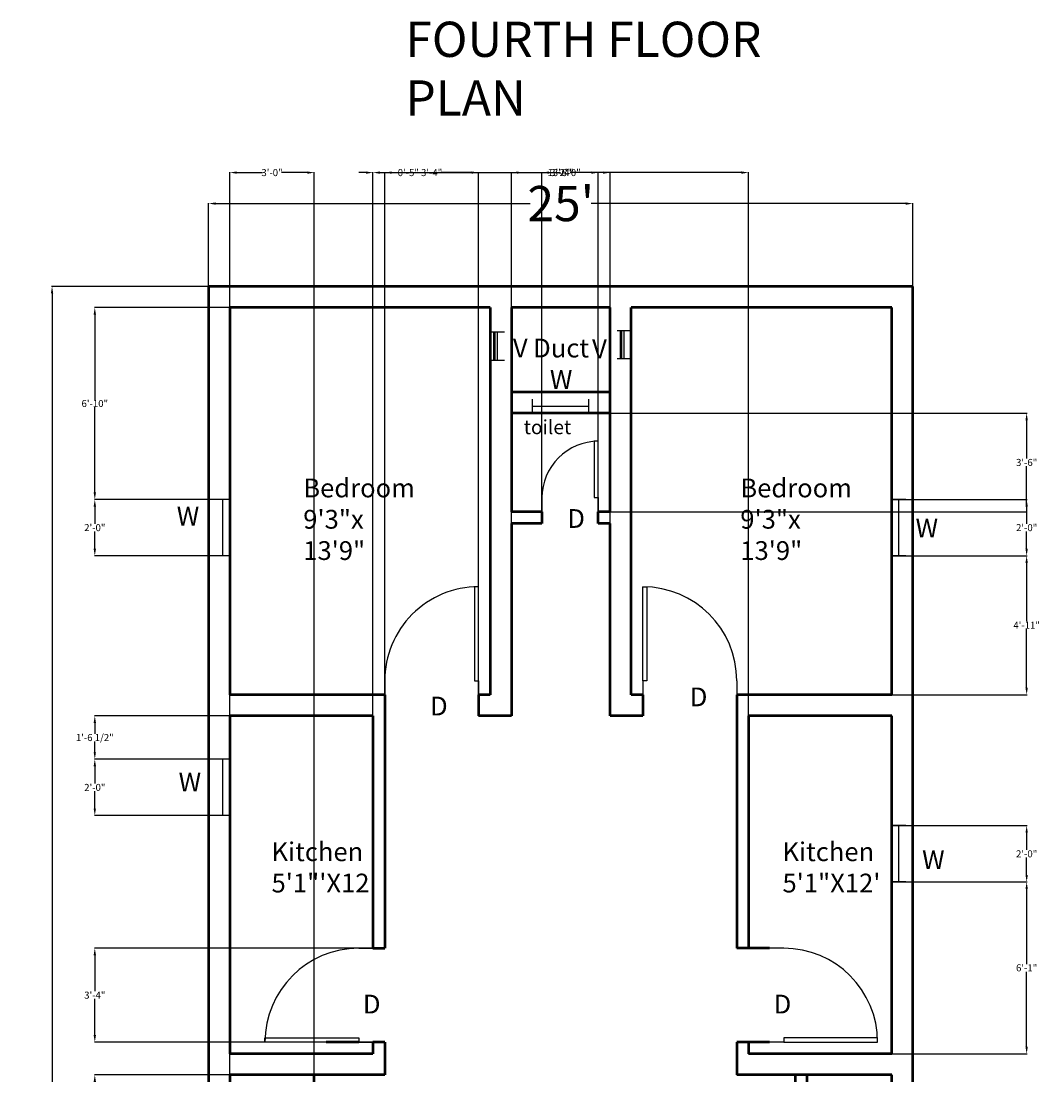
# Model space of a CAD drawing. Units: inches. Extents: x -250 to 2650, y 180 to 1183.
# Tile 10 of 10: x 2212 to 2646, y 734 to 1183. Entities that reach past the tile are written whole.
import ezdxf

# ---------------------------------------------------------------- set-up
doc = ezdxf.new("R2010")
doc.units = ezdxf.units.IN
doc.header["$MEASUREMENT"] = 0
for name, color, linetype, lineweight in [('A-ANNO-DIMS', 2, 'Continuous', 18), ('A-ANNO-TEXT', 7, 'Continuous', 18), ('A-AREA-IDEN', 3, 'Continuous', 18), ('A-DOOR', 4, 'Continuous', 25), ('A-GLAZ', 3, 'Continuous', 25), ('A-WALL', 7, 'Continuous', 50)]:
    doc.layers.add(name, color=color, linetype=linetype, lineweight=lineweight)
doc.styles.get("Standard").update_dxf_attribs({"font": 'arial.ttf'})
doc.dimstyles.get("Standard").update_dxf_attribs({"dimtxt": 3, "dimasz": 3, "dimexe": 0.18, "dimexo": 0.0625, "dimgap": 0.09, "dimtad": 0, "dimtih": 1, "dimtoh": 1, "dimdec": 0, "dimzin": 0, "dimdsep": 46, "dimlunit": 3, "dimtxsty": 'Standard', "dimcen": 0.09, "dimadec": 0, "dimazin": 0, "dimtfac": 1, "dimtdec": 0, "dimtofl": 0, "dimtmove": 0, "dimatfit": 3, "dimfxl": 1, "dimtolj": 1, "dimtzin": 0, "dimarcsym": 0})

# ---------------------------------------------------------------- blocks, each defined once
blk = doc.blocks.new('*D38')
at = {"layer": 'A-ANNO-DIMS', "color": 0, "lineweight": -2, "transparency": 16777216}
for p, q in [((2292.19, 1070.09), (2292.19, 1105.5)), ((2295.19, 1105.32), (2429.24, 1105.32)), ((2589.19, 1105.32), (2455.13, 1105.32)), ((2592.19, 1070.09), (2592.19, 1105.5))]:
    blk.add_line(p, q, dxfattribs=at)
at = {"layer": 'A-ANNO-DIMS', "color": 0, "transparency": 16777216}
for points in [[(2295.19, 1105.82), (2295.19, 1104.82), (2292.19, 1105.32)], [(2589.19, 1105.82), (2589.19, 1104.82), (2592.19, 1105.32)]]:
    blk.add_solid(points, dxfattribs=at)
at = {"layer": 'Defpoints', "color": 0, "transparency": 16777216}
for p in [(2292.19, 1105.32), (2292.19, 1070.02), (2592.19, 1070.02)]:
    blk.add_point(p, dxfattribs=at)
at = {"layer": 'A-ANNO-DIMS', "color": 0, "transparency": 16777216, "insert": (2442.19, 1105.32), "char_height": 3, "attachment_point": 5}
blk.add_mtext("\\A1;{\\H5x;25'}", dxfattribs=at)
blk = doc.blocks.new('*D39')
at = {"layer": 'A-ANNO-DIMS', "color": 0, "lineweight": -2, "transparency": 16777216}
for p, q in [((2292.12, 1070.02), (2225.3, 1070.02)), ((2225.48, 1067.02), (2225.48, 657.77)), ((2225.48, 233.02), (2225.48, 642.28)), ((2292.12, 230.02), (2225.3, 230.02))]:
    blk.add_line(p, q, dxfattribs=at)
at = {"layer": 'A-ANNO-DIMS', "color": 0, "transparency": 16777216}
for points in [[(2224.98, 1067.02), (2225.98, 1067.02), (2225.48, 1070.02)], [(2224.98, 233.02), (2225.98, 233.02), (2225.48, 230.02)]]:
    blk.add_solid(points, dxfattribs=at)
at = {"layer": 'Defpoints', "color": 0, "transparency": 16777216}
for p in [(2292.19, 1070.02), (2225.48, 230.02), (2292.19, 230.02)]:
    blk.add_point(p, dxfattribs=at)
at = {"layer": 'A-ANNO-DIMS', "color": 0, "transparency": 16777216, "insert": (2225.48, 650.02), "char_height": 3, "attachment_point": 5}
blk.add_mtext("\\A1;{\\H5x;70'}", dxfattribs=at)
blk = doc.blocks.new('*U24')
for p, q in [((-24, 6), (-24, 0)), ((0, 6), (0, 0)), ((0, 3), (-24, 3))]:
    blk.add_line(p, q)
blk = doc.blocks.new('*U23')
for p, q in [((-24, 6), (-24, 0)), ((0, 6), (0, 0)), ((0, 3), (-24, 3))]:
    blk.add_line(p, q)
blk = doc.blocks.new('*U22')
for p, q in [((0, 6), (0, 0)), ((12, 6), (12, 0)), ((0, 3), (12, 3))]:
    blk.add_line(p, q)
blk = doc.blocks.new('*U26')
for p, q in [((-40, 0), (-40, -6)), ((0, 0), (0, -6))]:
    blk.add_line(p, q)
blk.add_lwpolyline([(0, 0), (0, 40), (-1.75, 40), (-1.75, 0)], close=True)
blk.add_arc((0, 0), 40, 90, 180)
blk = doc.blocks.new('*U44')
for p, q in [((0, 0), (0, 6)), ((40, 0), (40, 6))]:
    blk.add_line(p, q)
blk.add_lwpolyline([(0, 0), (0, -40), (1.75, -40), (1.75, 0)], close=True)
blk.add_arc((0, 0), 40, 270, 0)
blk = doc.blocks.new('*U45')
for p, q in [((-40, 0), (-40, 6)), ((0, 0), (0, 6))]:
    blk.add_line(p, q)
blk.add_lwpolyline([(0, 0), (0, -40), (-1.75, -40), (-1.75, 0)], close=True)
blk.add_arc((0, 0), 40, 180, 270)
blk = doc.blocks.new('*U46')
for p, q in [((-24, 6), (-24, 0)), ((0, 6), (0, 0)), ((0, 3), (-24, 3))]:
    blk.add_line(p, q)
blk = doc.blocks.new('*U47')
for p, q in [((-40, 0), (-40, 6)), ((0, 0), (0, 6))]:
    blk.add_line(p, q)
blk.add_lwpolyline([(0, 0), (0, -40), (-1.75, -40), (-1.75, 0)], close=True)
blk.add_arc((0, 0), 40, 180, 270)
blk = doc.blocks.new('*U48')
for p, q in [((0, 0), (0, 6)), ((24, 0), (24, 6))]:
    blk.add_line(p, q)
blk.add_lwpolyline([(0, 0), (0, -24), (1.75, -24), (1.75, 0)], close=True)
blk.add_arc((0, 0), 24, 270, 0)
blk = doc.blocks.new('*D175')
at = {"layer": 'A-ANNO-DIMS', "color": 0, "lineweight": -2, "transparency": 16777216}
for p, q in [((2301.19, 734.09), (2301.19, 1118.7)), ((2304.19, 1118.52), (2315.11, 1118.52)), ((2334.19, 1118.52), (2323.26, 1118.52)), ((2337.19, 734.09), (2337.19, 1118.7))]:
    blk.add_line(p, q, dxfattribs=at)
at = {"layer": 'A-ANNO-DIMS', "color": 0, "transparency": 16777216}
for points in [[(2304.19, 1119.02), (2304.19, 1118.02), (2301.19, 1118.52)], [(2334.19, 1119.02), (2334.19, 1118.02), (2337.19, 1118.52)]]:
    blk.add_solid(points, dxfattribs=at)
at = {"layer": 'Defpoints', "color": 0, "transparency": 16777216}
for p in [(2337.19, 1118.52), (2301.19, 734.02), (2337.19, 734.02)]:
    blk.add_point(p, dxfattribs=at)
at = {"layer": 'A-ANNO-DIMS', "color": 0, "transparency": 16777216, "insert": (2319.19, 1118.52), "char_height": 3, "attachment_point": 5}
blk.add_mtext('\\A1;3\'-0"', dxfattribs=at)
blk = doc.blocks.new('*D177')
at = {"layer": 'A-ANNO-DIMS', "color": 0, "lineweight": -2, "transparency": 16777216}
for p, q in [((2301.12, 734.02), (2243.51, 734.02)), ((2243.69, 731.02), (2243.69, 717.09)), ((2243.69, 699.91), (2243.69, 713.84)), ((2301.12, 696.91), (2243.51, 696.91))]:
    blk.add_line(p, q, dxfattribs=at)
at = {"layer": 'A-ANNO-DIMS', "color": 0, "transparency": 16777216}
for points in [[(2243.19, 731.02), (2244.19, 731.02), (2243.69, 734.02)], [(2243.19, 699.91), (2244.19, 699.91), (2243.69, 696.91)]]:
    blk.add_solid(points, dxfattribs=at)
at = {"layer": 'Defpoints', "color": 0, "transparency": 16777216}
for p in [(2243.69, 734.02), (2301.19, 734.02), (2301.19, 696.91)]:
    blk.add_point(p, dxfattribs=at)
at = {"layer": 'A-ANNO-DIMS', "color": 0, "transparency": 16777216, "insert": (2243.69, 715.47), "char_height": 3, "attachment_point": 5}
blk.add_mtext('\\A1;3\'-1"', dxfattribs=at)
blk = doc.blocks.new('*D185')
at = {"layer": 'A-ANNO-DIMS', "color": 0, "lineweight": -2, "transparency": 16777216}
for p, q in [((2421.19, 969.09), (2421.19, 1118.7)), ((2424.19, 1118.52), (2438.11, 1118.52)), ((2460.19, 1118.52), (2446.26, 1118.52)), ((2463.19, 969.09), (2463.19, 1118.7))]:
    blk.add_line(p, q, dxfattribs=at)
at = {"layer": 'A-ANNO-DIMS', "color": 0, "transparency": 16777216}
for points in [[(2424.19, 1119.02), (2424.19, 1118.02), (2421.19, 1118.52)], [(2460.19, 1119.02), (2460.19, 1118.02), (2463.19, 1118.52)]]:
    blk.add_solid(points, dxfattribs=at)
at = {"layer": 'Defpoints', "color": 0, "transparency": 16777216}
for p in [(2463.19, 1118.52), (2421.19, 969.02), (2463.19, 969.02)]:
    blk.add_point(p, dxfattribs=at)
at = {"layer": 'A-ANNO-DIMS', "color": 0, "transparency": 16777216, "insert": (2442.19, 1118.52), "char_height": 3, "attachment_point": 5}
blk.add_mtext('\\A1;3\'-6"', dxfattribs=at)
blk = doc.blocks.new('*D186')
at = {"layer": 'A-ANNO-DIMS', "color": 0, "lineweight": -2, "transparency": 16777216}
for p, q in [((2463.25, 1016.02), (2640.87, 1016.02)), ((2640.69, 1013.02), (2640.69, 996.65)), ((2640.69, 977.02), (2640.69, 993.4)), ((2463.25, 974.02), (2640.87, 974.02))]:
    blk.add_line(p, q, dxfattribs=at)
at = {"layer": 'A-ANNO-DIMS', "color": 0, "transparency": 16777216}
for points in [[(2640.19, 1013.02), (2641.19, 1013.02), (2640.69, 1016.02)], [(2640.19, 977.02), (2641.19, 977.02), (2640.69, 974.02)]]:
    blk.add_solid(points, dxfattribs=at)
at = {"layer": 'Defpoints', "color": 0, "transparency": 16777216}
for p in [(2463.19, 1016.02), (2463.19, 974.02), (2640.69, 974.02)]:
    blk.add_point(p, dxfattribs=at)
at = {"layer": 'A-ANNO-DIMS', "color": 0, "transparency": 16777216, "insert": (2640.69, 995.02), "char_height": 3, "attachment_point": 5}
blk.add_mtext('\\A1;3\'-6"', dxfattribs=at)
blk = doc.blocks.new('*D187')
at = {"layer": 'A-ANNO-DIMS', "color": 0, "lineweight": -2, "transparency": 16777216}
for p, q in [((2434.19, 974.09), (2434.19, 1118.7)), ((2437.19, 1118.52), (2442.08, 1118.52)), ((2455.19, 1118.52), (2450.29, 1118.52)), ((2458.19, 974.09), (2458.19, 1118.7))]:
    blk.add_line(p, q, dxfattribs=at)
at = {"layer": 'A-ANNO-DIMS', "color": 0, "transparency": 16777216}
for points in [[(2437.19, 1119.02), (2437.19, 1118.02), (2434.19, 1118.52)], [(2455.19, 1119.02), (2455.19, 1118.02), (2458.19, 1118.52)]]:
    blk.add_solid(points, dxfattribs=at)
at = {"layer": 'Defpoints', "color": 0, "transparency": 16777216}
for p in [(2458.19, 1118.52), (2434.19, 974.02), (2458.19, 974.02)]:
    blk.add_point(p, dxfattribs=at)
at = {"layer": 'A-ANNO-DIMS', "color": 0, "transparency": 16777216, "insert": (2446.19, 1118.52), "char_height": 3, "attachment_point": 5}
blk.add_mtext('\\A1;2\'-0"', dxfattribs=at)
blk = doc.blocks.new('*D188')
at = {"layer": 'A-ANNO-DIMS', "color": 0, "lineweight": -2, "transparency": 16777216}
for p, q in [((2367.19, 896.09), (2367.19, 1118.7)), ((2370.19, 1118.52), (2383.11, 1118.52)), ((2404.19, 1118.52), (2391.26, 1118.52)), ((2407.19, 896.09), (2407.19, 1118.7))]:
    blk.add_line(p, q, dxfattribs=at)
at = {"layer": 'A-ANNO-DIMS', "color": 0, "transparency": 16777216}
for points in [[(2370.19, 1119.02), (2370.19, 1118.02), (2367.19, 1118.52)], [(2404.19, 1119.02), (2404.19, 1118.02), (2407.19, 1118.52)]]:
    blk.add_solid(points, dxfattribs=at)
at = {"layer": 'Defpoints', "color": 0, "transparency": 16777216}
for p in [(2407.19, 1118.52), (2367.19, 896.02), (2407.19, 896.02)]:
    blk.add_point(p, dxfattribs=at)
at = {"layer": 'A-ANNO-DIMS', "color": 0, "transparency": 16777216, "insert": (2387.19, 1118.52), "char_height": 3, "attachment_point": 5}
blk.add_mtext('\\A1;3\'-4"', dxfattribs=at)
blk = doc.blocks.new('*D189')
at = {"layer": 'A-ANNO-DIMS', "color": 0, "lineweight": -2, "transparency": 16777216}
for p, q in [((2359.19, 1118.52), (2356.19, 1118.52)), ((2362.19, 788.09), (2362.19, 1118.7)), ((2367.19, 788.09), (2367.19, 1118.7)), ((2370.19, 1118.52), (2373.19, 1118.52))]:
    blk.add_line(p, q, dxfattribs=at)
at = {"layer": 'A-ANNO-DIMS', "color": 0, "transparency": 16777216}
for points in [[(2359.19, 1119.02), (2359.19, 1118.02), (2362.19, 1118.52)], [(2370.19, 1119.02), (2370.19, 1118.02), (2367.19, 1118.52)]]:
    blk.add_solid(points, dxfattribs=at)
at = {"layer": 'Defpoints', "color": 0, "transparency": 16777216}
for p in [(2367.19, 1118.52), (2362.19, 788.02), (2367.19, 788.02)]:
    blk.add_point(p, dxfattribs=at)
at = {"layer": 'A-ANNO-DIMS', "color": 0, "transparency": 16777216, "insert": (2377.26, 1118.52), "char_height": 3, "attachment_point": 5}
blk.add_mtext('\\A1;0\'-5"', dxfattribs=at)
blk = doc.blocks.new('*D190')
at = {"layer": 'A-ANNO-DIMS', "color": 0, "lineweight": -2, "transparency": 16777216}
for p, q in [((2362.19, 887.09), (2362.19, 1118.7)), ((2365.19, 1118.52), (2437.08, 1118.52)), ((2519.18, 1118.52), (2447.29, 1118.52)), ((2522.18, 887.09), (2522.18, 1118.7))]:
    blk.add_line(p, q, dxfattribs=at)
at = {"layer": 'A-ANNO-DIMS', "color": 0, "transparency": 16777216}
for points in [[(2365.19, 1119.02), (2365.19, 1118.02), (2362.19, 1118.52)], [(2519.18, 1119.02), (2519.18, 1118.02), (2522.18, 1118.52)]]:
    blk.add_solid(points, dxfattribs=at)
at = {"layer": 'Defpoints', "color": 0, "transparency": 16777216}
for p in [(2522.18, 1118.52), (2362.19, 887.02), (2522.18, 887.02)]:
    blk.add_point(p, dxfattribs=at)
at = {"layer": 'A-ANNO-DIMS', "color": 0, "transparency": 16777216, "insert": (2442.18, 1118.52), "char_height": 3, "attachment_point": 5}
blk.add_mtext('\\A1;13\'-4"', dxfattribs=at)
blk = doc.blocks.new('*D191')
at = {"layer": 'A-ANNO-DIMS', "color": 0, "lineweight": -2, "transparency": 16777216}
for p, q in [((2367.12, 788.02), (2243.51, 788.02)), ((2243.69, 785.02), (2243.69, 769.65)), ((2243.69, 751.02), (2243.69, 766.4)), ((2367.12, 748.02), (2243.51, 748.02))]:
    blk.add_line(p, q, dxfattribs=at)
at = {"layer": 'A-ANNO-DIMS', "color": 0, "transparency": 16777216}
for points in [[(2243.19, 785.02), (2244.19, 785.02), (2243.69, 788.02)], [(2243.19, 751.02), (2244.19, 751.02), (2243.69, 748.02)]]:
    blk.add_solid(points, dxfattribs=at)
at = {"layer": 'Defpoints', "color": 0, "transparency": 16777216}
for p in [(2243.69, 788.02), (2367.19, 788.02), (2367.19, 748.02)]:
    blk.add_point(p, dxfattribs=at)
at = {"layer": 'A-ANNO-DIMS', "color": 0, "transparency": 16777216, "insert": (2243.69, 768.02), "char_height": 3, "attachment_point": 5}
blk.add_mtext('\\A1;3\'-4"', dxfattribs=at)
blk = doc.blocks.new('*D192')
at = {"layer": 'A-ANNO-DIMS', "color": 0, "lineweight": -2, "transparency": 16777216}
for p, q in [((2301.12, 979.23), (2243.51, 979.23)), ((2243.69, 976.23), (2243.69, 968.85)), ((2243.69, 958.23), (2243.69, 965.61)), ((2301.12, 955.23), (2243.51, 955.23))]:
    blk.add_line(p, q, dxfattribs=at)
at = {"layer": 'A-ANNO-DIMS', "color": 0, "transparency": 16777216}
for points in [[(2243.19, 976.23), (2244.19, 976.23), (2243.69, 979.23)], [(2243.19, 958.23), (2244.19, 958.23), (2243.69, 955.23)]]:
    blk.add_solid(points, dxfattribs=at)
at = {"layer": 'Defpoints', "color": 0, "transparency": 16777216}
for p in [(2243.69, 979.23), (2301.19, 979.23), (2301.19, 955.23)]:
    blk.add_point(p, dxfattribs=at)
at = {"layer": 'A-ANNO-DIMS', "color": 0, "transparency": 16777216, "insert": (2243.69, 967.23), "char_height": 3, "attachment_point": 5}
blk.add_mtext('\\A1;2\'-0"', dxfattribs=at)
blk = doc.blocks.new('*D193')
at = {"layer": 'A-ANNO-DIMS', "color": 0, "lineweight": -2, "transparency": 16777216}
for p, q in [((2301.12, 1061.02), (2243.51, 1061.02)), ((2243.69, 1058.02), (2243.69, 1021.75)), ((2243.69, 982.23), (2243.69, 1018.51)), ((2301.12, 979.23), (2243.51, 979.23))]:
    blk.add_line(p, q, dxfattribs=at)
at = {"layer": 'A-ANNO-DIMS', "color": 0, "transparency": 16777216}
for points in [[(2243.19, 1058.02), (2244.19, 1058.02), (2243.69, 1061.02)], [(2243.19, 982.23), (2244.19, 982.23), (2243.69, 979.23)]]:
    blk.add_solid(points, dxfattribs=at)
at = {"layer": 'Defpoints', "color": 0, "transparency": 16777216}
for p in [(2243.69, 1061.02), (2301.19, 1061.02), (2301.19, 979.23)]:
    blk.add_point(p, dxfattribs=at)
at = {"layer": 'A-ANNO-DIMS', "color": 0, "transparency": 16777216, "insert": (2243.69, 1020.13), "char_height": 3, "attachment_point": 5}
blk.add_mtext('\\A1;6\'-10"', dxfattribs=at)
blk = doc.blocks.new('*D194')
at = {"layer": 'A-ANNO-DIMS', "color": 0, "lineweight": -2, "transparency": 16777216}
for p, q in [((2301.12, 868.53), (2243.51, 868.53)), ((2243.69, 865.53), (2243.69, 858.15)), ((2243.69, 847.53), (2243.69, 854.91)), ((2301.12, 844.53), (2243.51, 844.53))]:
    blk.add_line(p, q, dxfattribs=at)
at = {"layer": 'A-ANNO-DIMS', "color": 0, "transparency": 16777216}
for points in [[(2243.19, 865.53), (2244.19, 865.53), (2243.69, 868.53)], [(2243.19, 847.53), (2244.19, 847.53), (2243.69, 844.53)]]:
    blk.add_solid(points, dxfattribs=at)
at = {"layer": 'Defpoints', "color": 0, "transparency": 16777216}
for p in [(2243.69, 868.53), (2301.19, 868.53), (2301.19, 844.53)]:
    blk.add_point(p, dxfattribs=at)
at = {"layer": 'A-ANNO-DIMS', "color": 0, "transparency": 16777216, "insert": (2243.69, 856.53), "char_height": 3, "attachment_point": 5}
blk.add_mtext('\\A1;2\'-0"', dxfattribs=at)
blk = doc.blocks.new('*D195')
at = {"layer": 'A-ANNO-DIMS', "color": 0, "lineweight": -2, "transparency": 16777216}
for p, q in [((2301.12, 887.02), (2243.51, 887.02)), ((2243.69, 884.02), (2243.69, 879.42)), ((2243.69, 871.53), (2243.69, 876.14)), ((2301.12, 868.53), (2243.51, 868.53))]:
    blk.add_line(p, q, dxfattribs=at)
at = {"layer": 'A-ANNO-DIMS', "color": 0, "transparency": 16777216}
for points in [[(2243.19, 884.02), (2244.19, 884.02), (2243.69, 887.02)], [(2243.19, 871.53), (2244.19, 871.53), (2243.69, 868.53)]]:
    blk.add_solid(points, dxfattribs=at)
at = {"layer": 'Defpoints', "color": 0, "transparency": 16777216}
for p in [(2243.69, 887.02), (2301.19, 887.02), (2301.19, 868.53)]:
    blk.add_point(p, dxfattribs=at)
at = {"layer": 'A-ANNO-DIMS', "color": 0, "transparency": 16777216, "insert": (2243.69, 877.78), "char_height": 3, "attachment_point": 5}
blk.add_mtext('\\A1;1\'-6 1/2"', dxfattribs=at)
blk = doc.blocks.new('*D196')
at = {"layer": 'A-ANNO-DIMS', "color": 0, "lineweight": -2, "transparency": 16777216}
for p, q in [((2583.25, 979.23), (2640.87, 979.23)), ((2640.69, 976.23), (2640.69, 968.85)), ((2640.69, 958.23), (2640.69, 965.61)), ((2583.25, 955.23), (2640.87, 955.23))]:
    blk.add_line(p, q, dxfattribs=at)
at = {"layer": 'A-ANNO-DIMS', "color": 0, "transparency": 16777216}
for points in [[(2640.19, 976.23), (2641.19, 976.23), (2640.69, 979.23)], [(2640.19, 958.23), (2641.19, 958.23), (2640.69, 955.23)]]:
    blk.add_solid(points, dxfattribs=at)
at = {"layer": 'Defpoints', "color": 0, "transparency": 16777216}
for p in [(2583.19, 979.23), (2640.69, 979.23), (2583.19, 955.23)]:
    blk.add_point(p, dxfattribs=at)
at = {"layer": 'A-ANNO-DIMS', "color": 0, "transparency": 16777216, "insert": (2640.69, 967.23), "char_height": 3, "attachment_point": 5}
blk.add_mtext('\\A1;2\'-0"', dxfattribs=at)
blk = doc.blocks.new('*D197')
at = {"layer": 'A-ANNO-DIMS', "color": 0, "lineweight": -2, "transparency": 16777216}
for p, q in [((2583.25, 955.23), (2640.87, 955.23)), ((2640.69, 952.23), (2640.69, 927.22)), ((2640.69, 899.02), (2640.69, 924.03)), ((2583.25, 896.02), (2640.87, 896.02))]:
    blk.add_line(p, q, dxfattribs=at)
at = {"layer": 'A-ANNO-DIMS', "color": 0, "transparency": 16777216}
for points in [[(2640.19, 952.23), (2641.19, 952.23), (2640.69, 955.23)], [(2640.19, 899.02), (2641.19, 899.02), (2640.69, 896.02)]]:
    blk.add_solid(points, dxfattribs=at)
at = {"layer": 'Defpoints', "color": 0, "transparency": 16777216}
for p in [(2583.19, 955.23), (2640.69, 955.23), (2583.19, 896.02)]:
    blk.add_point(p, dxfattribs=at)
at = {"layer": 'A-ANNO-DIMS', "color": 0, "transparency": 16777216, "insert": (2640.69, 925.63), "char_height": 3, "attachment_point": 5}
blk.add_mtext('\\A1;4\'-11"', dxfattribs=at)
blk = doc.blocks.new('*D198')
at = {"layer": 'A-ANNO-DIMS', "color": 0, "lineweight": -2, "transparency": 16777216}
for p, q in [((2583.25, 840.25), (2640.87, 840.25)), ((2640.69, 837.25), (2640.69, 829.87)), ((2640.69, 819.25), (2640.69, 826.63)), ((2583.25, 816.25), (2640.87, 816.25))]:
    blk.add_line(p, q, dxfattribs=at)
at = {"layer": 'A-ANNO-DIMS', "color": 0, "transparency": 16777216}
for points in [[(2640.19, 837.25), (2641.19, 837.25), (2640.69, 840.25)], [(2640.19, 819.25), (2641.19, 819.25), (2640.69, 816.25)]]:
    blk.add_solid(points, dxfattribs=at)
at = {"layer": 'Defpoints', "color": 0, "transparency": 16777216}
for p in [(2583.19, 840.25), (2640.69, 840.25), (2583.19, 816.25)]:
    blk.add_point(p, dxfattribs=at)
at = {"layer": 'A-ANNO-DIMS', "color": 0, "transparency": 16777216, "insert": (2640.69, 828.25), "char_height": 3, "attachment_point": 5}
blk.add_mtext('\\A1;2\'-0"', dxfattribs=at)
blk = doc.blocks.new('*D199')
at = {"layer": 'A-ANNO-DIMS', "color": 0, "lineweight": -2, "transparency": 16777216}
for p, q in [((2583.25, 816.25), (2640.87, 816.25)), ((2640.69, 813.25), (2640.69, 781.26)), ((2640.69, 746.02), (2640.69, 778.01)), ((2583.25, 743.02), (2640.87, 743.02))]:
    blk.add_line(p, q, dxfattribs=at)
at = {"layer": 'A-ANNO-DIMS', "color": 0, "transparency": 16777216}
for points in [[(2640.19, 813.25), (2641.19, 813.25), (2640.69, 816.25)], [(2640.19, 746.02), (2641.19, 746.02), (2640.69, 743.02)]]:
    blk.add_solid(points, dxfattribs=at)
at = {"layer": 'Defpoints', "color": 0, "transparency": 16777216}
for p in [(2583.19, 816.25), (2640.69, 816.25), (2583.19, 743.02)]:
    blk.add_point(p, dxfattribs=at)
at = {"layer": 'A-ANNO-DIMS', "color": 0, "transparency": 16777216, "insert": (2640.69, 779.64), "char_height": 3, "attachment_point": 5}
blk.add_mtext('\\A1;6\'-1"', dxfattribs=at)

msp = doc.modelspace()

# ---------------------------------------------------------------- linework, layer by layer
at = {"layer": 'A-WALL'}
for p, q in [((2592.19, 1070.02), (2292.19, 1070.02)), ((2292.19, 1070.02), (2292.19, 230.02)), ((2592.19, 230.02), (2592.19, 1070.02)), ((2301.19, 1061.02), (2301.19, 1025.02)), ((2301.19, 1061.02), (2301.19, 896.02)), ((2412.19, 1061.02), (2301.19, 1061.02)), ((2412.19, 1061.02), (2412.19, 896.02)), ((2424.19, 1061.02), (2421.19, 1061.02)), ((2421.19, 1061.02), (2421.19, 974.02)), ((2460.19, 1061.02), (2424.19, 1061.02)), ((2463.19, 1061.02), (2460.19, 1061.02)), ((2463.19, 974.02), (2463.19, 1061.02)), ((2583.19, 1061.02), (2472.19, 1061.02)), ((2472.19, 896.02), (2472.19, 1061.02)), ((2583.19, 1025.02), (2583.19, 1061.02)), ((2583.19, 1025.02), (2583.19, 1061.02)), ((2583.19, 896.02), (2583.19, 1061.02)), ((2583.19, 1025.02), (2583.19, 1061.02)), ((2583.19, 1025.02), (2583.19, 1061.02)), ((2467.92, 1039.26), (2467.92, 1051.26)), ((2413.93, 1038.66), (2413.93, 1050.66)), ((2463.19, 1025.02), (2421.19, 1025.02)), ((2463.19, 1016.02), (2421.19, 1016.02)), ((2583.19, 896.02), (2583.19, 1016.02)), ((2583.19, 896.02), (2583.19, 1016.02)), ((2434.19, 974.02), (2421.19, 974.02)), ((2434.19, 974.02), (2434.19, 969.02)), ((2463.19, 974.02), (2458.19, 974.02)), ((2458.19, 969.02), (2458.19, 974.02)), ((2421.19, 969.02), (2421.19, 887.02)), ((2434.19, 969.02), (2421.19, 969.02)), ((2463.19, 969.02), (2458.19, 969.02)), ((2463.19, 887.02), (2463.19, 969.02)), ((2367.19, 896.02), (2301.19, 896.02)), ((2367.19, 896.02), (2367.19, 788.02)), ((2412.19, 896.02), (2407.19, 896.02)), ((2407.19, 896.02), (2407.19, 887.02)), ((2477.19, 896.02), (2472.19, 896.02)), ((2477.19, 896.02), (2477.19, 887.02)), ((2583.19, 896.02), (2517.18, 896.02)), ((2517.18, 896.02), (2517.18, 788.02)), ((2301.19, 887.02), (2301.19, 743.02)), ((2362.19, 887.02), (2301.19, 887.02)), ((2362.19, 887.02), (2362.19, 788.02)), ((2421.19, 887.02), (2407.19, 887.02)), ((2477.19, 887.02), (2463.19, 887.02)), ((2583.19, 887.02), (2522.18, 887.02)), ((2522.18, 887.02), (2522.18, 788.02)), ((2583.19, 743.02), (2583.19, 887.02)), ((2583.19, 743.02), (2583.19, 887.02)), ((2583.19, 743.02), (2583.19, 887.02)), ((2362.19, 788.02), (2367.19, 788.02)), ((2531.18, 788.02), (2517.18, 788.02)), ((2356.19, 748.02), (2342.19, 748.02)), ((2367.19, 748.02), (2362.19, 748.02)), ((2362.19, 748.02), (2362.19, 743.02)), ((2367.19, 748.02), (2367.19, 734.02)), ((2531.18, 748.02), (2517.18, 748.02)), ((2517.18, 748.02), (2517.18, 734.02)), ((2522.18, 748.02), (2522.18, 743.02)), ((2362.19, 743.02), (2301.19, 743.02)), ((2583.19, 743.02), (2522.18, 743.02)), ((2367.19, 734.02), (2301.19, 734.02)), ((2301.19, 734.02), (2301.19, 696.91)), ((2337.19, 696.91), (2337.19, 734.02)), ((2583.19, 734.02), (2517.18, 734.02)), ((2542.19, 686.91), (2542.19, 734.02)), ((2542.19, 686.91), (2542.19, 734.02)), ((2547.19, 696.91), (2547.19, 734.02)), ((2583.19, 696.91), (2583.19, 734.02)), ((2583.19, 716.02), (2583.19, 734.02))]:
    msp.add_line(p, q, dxfattribs=at)

# ---------------------------------------------------------------- block references
at = {"layer": 'A-DOOR'}
for name, p, rotation in [('*U48', (2458.19, 980.02), 180), ('*U44', (2407.19, 902.02), 180), ('*U45', (2477.18, 902.02), 180), ('*U47', (2356.19, 748.02), 270), ('*U26', (2537.18, 748.02), 270)]:
    msp.add_blockref(name, p, dxfattribs=dict(at, rotation=rotation))
at = {"layer": 'A-GLAZ'}
for name, p, rotation in [('*U22', (2472.19, 1039.26), 89.99999999999996), ('*U22', (2418.19, 1038.66), 89.99999999999996), ('*U46', (2430.11, 1022.02), 180), ('*U23', (2295.19, 955.23), 270), ('*U24', (2583.19, 955.23), 270), ('*U23', (2295.19, 844.53), 270), ('*U24', (2583.19, 816.25), 270)]:
    msp.add_blockref(name, p, dxfattribs=dict(at, rotation=rotation))

# ---------------------------------------------------------------- texts
at = {"layer": 'A-ANNO-TEXT', "attachment_point": 1}
for s, width, insert, char_height in [('FOURTH FLOOR PLAN ', 207.4062, (2375.99, 1182.82), 15), ('V', 10.3916, (2421.82, 1047.78), 8), ('V', 10.3916, (2455.56, 1047.43), 8), ('W', 10.3916, (2437.57, 1034.36), 8), ('W', 10.3916, (2278.6, 976.14), 8), ('D', 10.3916, (2444.99, 975.12), 8), ('W', 10.3916, (2593.37, 971.03), 8), ('D', 10.3916, (2497.18, 899.11), 8), ('D', 10.3916, (2386.53, 895.2), 8), ('W', 10.3916, (2279.4, 862.8), 8), ('W', 10.3916, (2596.15, 829.71), 8), ('D', 10.3916, (2357.91, 768.2), 8), ('D', 10.3916, (2532.91, 768.2), 8)]:
    msp.add_mtext_dynamic_manual_height_columns(s, width=width, gutter_width=1, heights=[0], dxfattribs=dict(at, insert=insert, char_height=char_height))
at = {"layer": 'A-AREA-IDEN', "attachment_point": 1}
for s, width, heights, insert, char_height in [('{\\H2.66667x;Duct} ', 7.71, [3.05], (2430.44, 1047.76), 3), ('toilet', 19.3499, [0], (2426.42, 1013.06), 6), ('Bedroom \\P9\'3"x 13\'9"', 51.3886, [0], (2332.5, 988.13), 8), ('Bedroom \\P9\'3"x 13\'9"', 51.3886, [0], (2518.7, 988.13), 8), ('Kitchen 5\'1"\'X12\'', 37.1044, [0], (2318.99, 833.12), 8), ('Kitchen 5\'1"X12\'', 37.1044, [0], (2536.67, 833.12), 8)]:
    msp.add_mtext_dynamic_manual_height_columns(s, width=width, gutter_width=1, heights=heights, dxfattribs=dict(at, insert=insert, char_height=char_height))

# ---------------------------------------------------------------- dimensions: what is measured, and where the dimension line sits
at = {"layer": 'A-ANNO-DIMS'}
for base, p1, p2, picture, middle in [((2337.19, 1118.52), (2301.19, 734.02), (2337.19, 734.02), '*D175', (2319.19, 1118.52)), ((2367.19, 1118.52), (2362.19, 788.02), (2367.19, 788.02), '*D189', (2377.26, 1118.52)), ((2522.18, 1118.52), (2362.19, 887.02), (2522.18, 887.02), '*D190', (2442.18, 1118.52)), ((2407.19, 1118.52), (2367.19, 896.02), (2407.19, 896.02), '*D188', (2387.19, 1118.52)), ((2463.19, 1118.52), (2421.19, 969.02), (2463.19, 969.02), '*D185', (2442.19, 1118.52)), ((2458.19, 1118.52), (2434.19, 974.02), (2458.19, 974.02), '*D187', (2446.19, 1118.52))]:
    dim = msp.add_linear_dim(base=base, p1=p1, p2=p2, dimstyle='Standard', override={"dimdec": 1, "dimlfac": 1, "dimrnd": 0, "dimzin": 1, "dimdsep": 46, "dimlunit": 4, "dimfrac": 2}, dxfattribs=at)
    dim.commit()
    dim.dimension.update_dxf_attribs({"geometry": picture, "text_midpoint": middle})
dim = msp.add_linear_dim(base=(2292.19, 1105.32), p1=(2592.19, 1070.02), p2=(2292.19, 1070.02), text='{\\H5x;<>}', dimstyle='Standard', override={"dimclrd": 0, "dimclre": 0, "dimclrt": 0}, dxfattribs=at)
dim.commit()
dim.dimension.update_dxf_attribs({"geometry": '*D38', "text_midpoint": (2442.19, 1105.32)})
dim = msp.add_linear_dim(base=(2225.48, 230.02), p1=(2292.19, 1070.02), p2=(2292.19, 230.02), angle=90, text='{\\H5x;<>}', dimstyle='Standard', override={"dimclrd": 0, "dimclre": 0, "dimclrt": 0}, dxfattribs=at)
dim.commit()
dim.dimension.update_dxf_attribs({"geometry": '*D39', "text_midpoint": (2225.48, 650.02)})
for base, p1, p2, picture, middle in [((2243.69, 1061.02), (2301.19, 979.23), (2301.19, 1061.02), '*D193', (2243.69, 1020.13)), ((2640.69, 974.02), (2463.19, 1016.02), (2463.19, 974.02), '*D186', (2640.69, 995.02)), ((2243.69, 979.23), (2301.19, 955.23), (2301.19, 979.23), '*D192', (2243.69, 967.23)), ((2640.69, 979.23), (2583.19, 955.23), (2583.19, 979.23), '*D196', (2640.69, 967.23)), ((2640.69, 955.23), (2583.19, 896.02), (2583.19, 955.23), '*D197', (2640.69, 925.63)), ((2243.69, 887.02), (2301.19, 868.53), (2301.19, 887.02), '*D195', (2243.69, 877.78)), ((2243.69, 868.53), (2301.19, 844.53), (2301.19, 868.53), '*D194', (2243.69, 856.53)), ((2640.69, 840.25), (2583.19, 816.25), (2583.19, 840.25), '*D198', (2640.69, 828.25)), ((2640.69, 816.25), (2583.19, 743.02), (2583.19, 816.25), '*D199', (2640.69, 779.64)), ((2243.69, 788.02), (2367.19, 748.02), (2367.19, 788.02), '*D191', (2243.69, 768.02)), ((2243.69, 734.02), (2301.19, 696.91), (2301.19, 734.02), '*D177', (2243.69, 715.47))]:
    dim = msp.add_linear_dim(base=base, p1=p1, p2=p2, angle=90, dimstyle='Standard', override={"dimdec": 1, "dimlfac": 1, "dimrnd": 0, "dimzin": 1, "dimdsep": 46, "dimlunit": 4, "dimfrac": 2}, dxfattribs=at)
    dim.commit()
    dim.dimension.update_dxf_attribs({"geometry": picture, "text_midpoint": middle})

doc.saveas('drawing.dxf')
